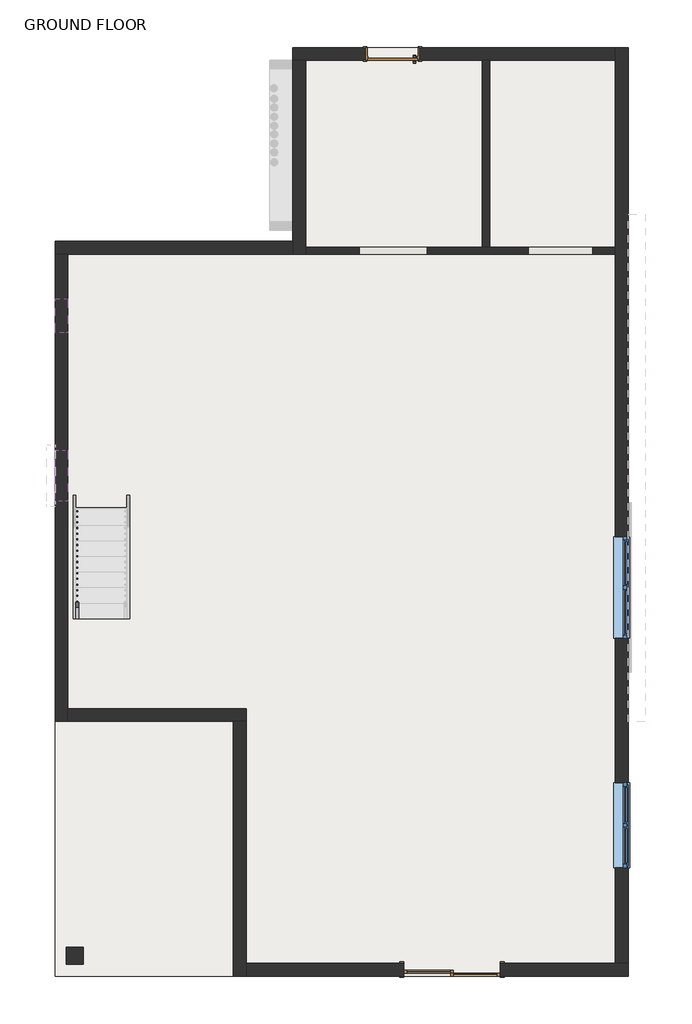
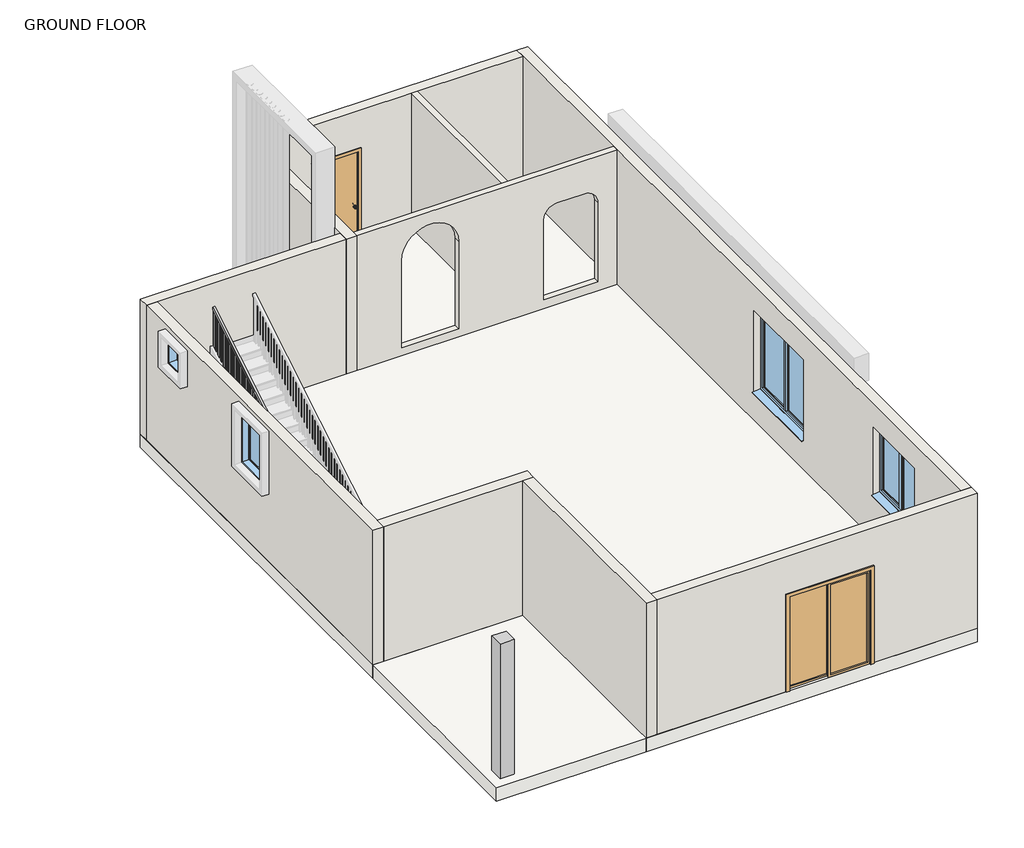
# One storey, part 1 of 2: 10 walls, 4 windows, 2 doors, 2 slabs, 1 column, 1 railing.
"""IFC4 building model written with IfcOpenShell, lengths in millimetres."""

from ifc_helpers import new_model, si_unit, frame, origin, origin_with_axes, place, context, project, spatial, polyline, circle_curve, outline, extrude, faceted_brep, transform, mapped, element, save
from ifc_brep_helpers import plane_surface, revolved_surface, advanced_brep
from components import rectangular_column_1_x_1_columns_77852fec, door_45189e27, door_1d7b229f, window_80340324, fixed_window_3_x_3_dcb239d8, w2_6_x_6_window_82e362f5, w2_windows_5_x_5_8ac21896

model = new_model("IFC4")

# Units and contexts
model_context = context("Model", 3, world=origin())
ifc_project = project(units=[si_unit("LENGTHUNIT", "METRE", prefix="MILLI")], contexts=[model_context])

# Site, building, storey
site = spatial("IfcSite", under=ifc_project)
building = spatial("IfcBuilding", under=site)
storey = spatial("IfcBuildingStorey", under=building, Name="GROUND FLOOR", Elevation=304.8)

# Column
placement = place(None, origin())
rectangular_column_1_x_1_columns_shape = rectangular_column_1_x_1_columns_77852fec(model_context)
element("IfcColumn", 1, ObjectType="Rectangular Column : 1' x 1' columns", at=placement, inside=storey, context=model_context, shape_type="MappedRepresentation", body=[
    mapped(rectangular_column_1_x_1_columns_shape, transform((-5747.4727592, -4033.4659376, 0.0), x_axis=(1.0, 0.0, 0.0), y_axis=(0.0, 1.0, 0.0), z_axis=(0.0, 0.0, 1.0))),
])

# Doors
door_shape = door_45189e27(model_context)
element("IfcDoor", 2, ObjectType="Door-Double-Sliding : 68\" x 84\"", at=placement, inside=storey, context=model_context, shape_type="MappedRepresentation", body=[
    mapped(door_shape, transform((1027.2719693, -4152.8358748, 304.8), x_axis=(-1.0, 0.0, 0.0), y_axis=(0.0, -1.0, 0.0), z_axis=(0.0, 0.0, 1.0))),
])
door_2_shape = door_1d7b229f(model_context)
element("IfcDoor", 3, ObjectType="Door-Interior-Single-Flush_Panel-Wood : 36\" x 84\"", at=placement, inside=storey, context=model_context, shape_type="MappedRepresentation", body=[
    mapped(door_2_shape, transform((-39.5280307, 12150.7891252, 304.8), x_axis=(-1.0, 0.0, 0.0), y_axis=(0.0, -1.0, 0.0), z_axis=(0.0, 0.0, 1.0))),
])

# Railing
element("IfcRailing", 4, ObjectType="Handrail - Rectangular", at=placement, inside=storey, context=model_context, shape_type="SweptSolid", body=[
    extrude(outline(polyline([(2020.7325341, 1329.1318731), (2020.7325341, 1388.5333333), (6770.5325341, 4267.2), (6770.5325341, 4207.7985397), (2020.7325341, 1329.1318731)])), frame((-5721.5875748, 0.0, 0.0), z_axis=(1.0, 0.0, 0.0), x_axis=(0.0, 1.0, 0.0)), (0.0, 0.0, 1.0), 50.8),
    extrude(outline(polyline([(6703.8575341, 4167.3894488), (6703.8575341, 3183.4666667), (6684.8075341, 3183.4666667), (6684.8075341, 4155.8439943), (6703.8575341, 4167.3894488)])), frame((-5705.7125748, 0.0, 0.0), z_axis=(1.0, 0.0, 0.0), x_axis=(0.0, 1.0, 0.0)), (0.0, 0.0, 1.0), 19.05),
    extrude(outline(polyline([(6602.2575341, 4105.8136913), (6602.2575341, 3183.4666667), (6583.2075341, 3183.4666667), (6583.2075341, 4094.2682367), (6602.2575341, 4105.8136913)])), frame((-5705.7125748, 0.0, 0.0), z_axis=(1.0, 0.0, 0.0), x_axis=(0.0, 1.0, 0.0)), (0.0, 0.0, 1.0), 19.05),
    extrude(outline(polyline([(6500.6575341, 4044.2379337), (6500.6575341, 3183.4666667), (6481.6075341, 3183.4666667), (6481.6075341, 4032.6924791), (6500.6575341, 4044.2379337)])), frame((-5705.7125748, 0.0, 0.0), z_axis=(1.0, 0.0, 0.0), x_axis=(0.0, 1.0, 0.0)), (0.0, 0.0, 1.0), 19.05),
    extrude(outline(polyline([(6399.0575341, 3982.6621761), (6399.0575341, 3014.1333333), (6380.0075341, 3014.1333333), (6380.0075341, 3971.1167216), (6399.0575341, 3982.6621761)])), frame((-5705.7125748, 0.0, 0.0), z_axis=(1.0, 0.0, 0.0), x_axis=(0.0, 1.0, 0.0)), (0.0, 0.0, 1.0), 19.05),
    extrude(outline(polyline([(6297.4575341, 3921.0864185), (6297.4575341, 3014.1333333), (6278.4075341, 3014.1333333), (6278.4075341, 3909.540964), (6297.4575341, 3921.0864185)])), frame((-5705.7125748, 0.0, 0.0), z_axis=(1.0, 0.0, 0.0), x_axis=(0.0, 1.0, 0.0)), (0.0, 0.0, 1.0), 19.05),
    extrude(outline(polyline([(6195.8575341, 3859.510661), (6195.8575341, 2844.8), (6176.8075341, 2844.8), (6176.8075341, 3847.9652064), (6195.8575341, 3859.510661)])), frame((-5705.7125748, 0.0, 0.0), z_axis=(1.0, 0.0, 0.0), x_axis=(0.0, 1.0, 0.0)), (0.0, 0.0, 1.0), 19.05),
    extrude(outline(polyline([(6094.2575341, 3797.9349034), (6094.2575341, 2844.8), (6075.2075341, 2844.8), (6075.2075341, 3786.3894488), (6094.2575341, 3797.9349034)])), frame((-5705.7125748, 0.0, 0.0), z_axis=(1.0, 0.0, 0.0), x_axis=(0.0, 1.0, 0.0)), (0.0, 0.0, 1.0), 19.05),
    extrude(outline(polyline([(5992.6575341, 3736.3591458), (5992.6575341, 2844.8), (5973.6075341, 2844.8), (5973.6075341, 3724.8136913), (5992.6575341, 3736.3591458)])), frame((-5705.7125748, 0.0, 0.0), z_axis=(1.0, 0.0, 0.0), x_axis=(0.0, 1.0, 0.0)), (0.0, 0.0, 1.0), 19.05),
    extrude(outline(polyline([(5891.0575341, 3674.7833882), (5891.0575341, 2675.4666667), (5872.0075341, 2675.4666667), (5872.0075341, 3663.2379337), (5891.0575341, 3674.7833882)])), frame((-5705.7125748, 0.0, 0.0), z_axis=(1.0, 0.0, 0.0), x_axis=(0.0, 1.0, 0.0)), (0.0, 0.0, 1.0), 19.05),
    extrude(outline(polyline([(5789.4575341, 3613.2076307), (5789.4575341, 2675.4666667), (5770.4075341, 2675.4666667), (5770.4075341, 3601.6621761), (5789.4575341, 3613.2076307)])), frame((-5705.7125748, 0.0, 0.0), z_axis=(1.0, 0.0, 0.0), x_axis=(0.0, 1.0, 0.0)), (0.0, 0.0, 1.0), 19.05),
    extrude(outline(polyline([(5687.8575341, 3551.6318731), (5687.8575341, 2675.4666667), (5668.8075341, 2675.4666667), (5668.8075341, 3540.0864185), (5687.8575341, 3551.6318731)])), frame((-5705.7125748, 0.0, 0.0), z_axis=(1.0, 0.0, 0.0), x_axis=(0.0, 1.0, 0.0)), (0.0, 0.0, 1.0), 19.05),
    extrude(outline(polyline([(5586.2575341, 3490.0561155), (5586.2575341, 2506.1333333), (5567.2075341, 2506.1333333), (5567.2075341, 3478.510661), (5586.2575341, 3490.0561155)])), frame((-5705.7125748, 0.0, 0.0), z_axis=(1.0, 0.0, 0.0), x_axis=(0.0, 1.0, 0.0)), (0.0, 0.0, 1.0), 19.05),
    extrude(outline(polyline([(5484.6575341, 3428.4803579), (5484.6575341, 2506.1333333), (5465.6075341, 2506.1333333), (5465.6075341, 3416.9349034), (5484.6575341, 3428.4803579)])), frame((-5705.7125748, 0.0, 0.0), z_axis=(1.0, 0.0, 0.0), x_axis=(0.0, 1.0, 0.0)), (0.0, 0.0, 1.0), 19.05),
    extrude(outline(polyline([(5383.0575341, 3366.9046004), (5383.0575341, 2506.1333333), (5364.0075341, 2506.1333333), (5364.0075341, 3355.3591458), (5383.0575341, 3366.9046004)])), frame((-5705.7125748, 0.0, 0.0), z_axis=(1.0, 0.0, 0.0), x_axis=(0.0, 1.0, 0.0)), (0.0, 0.0, 1.0), 19.05),
    extrude(outline(polyline([(5281.4575341, 3305.3288428), (5281.4575341, 2336.8), (5262.4075341, 2336.8), (5262.4075341, 3293.7833882), (5281.4575341, 3305.3288428)])), frame((-5705.7125748, 0.0, 0.0), z_axis=(1.0, 0.0, 0.0), x_axis=(0.0, 1.0, 0.0)), (0.0, 0.0, 1.0), 19.05),
    extrude(outline(polyline([(5179.8575341, 3243.7530852), (5179.8575341, 2336.8), (5160.8075341, 2336.8), (5160.8075341, 3232.2076307), (5179.8575341, 3243.7530852)])), frame((-5705.7125748, 0.0, 0.0), z_axis=(1.0, 0.0, 0.0), x_axis=(0.0, 1.0, 0.0)), (0.0, 0.0, 1.0), 19.05),
    extrude(outline(polyline([(5078.2575341, 3182.1773276), (5078.2575341, 2167.4666667), (5059.2075341, 2167.4666667), (5059.2075341, 3170.6318731), (5078.2575341, 3182.1773276)])), frame((-5705.7125748, 0.0, 0.0), z_axis=(1.0, 0.0, 0.0), x_axis=(0.0, 1.0, 0.0)), (0.0, 0.0, 1.0), 19.05),
    extrude(outline(polyline([(4976.6575341, 3120.60157), (4976.6575341, 2167.4666667), (4957.6075341, 2167.4666667), (4957.6075341, 3109.0561155), (4976.6575341, 3120.60157)])), frame((-5705.7125748, 0.0, 0.0), z_axis=(1.0, 0.0, 0.0), x_axis=(0.0, 1.0, 0.0)), (0.0, 0.0, 1.0), 19.05),
    extrude(outline(polyline([(4875.0575341, 3059.0258125), (4875.0575341, 2167.4666667), (4856.0075341, 2167.4666667), (4856.0075341, 3047.4803579), (4875.0575341, 3059.0258125)])), frame((-5705.7125748, 0.0, 0.0), z_axis=(1.0, 0.0, 0.0), x_axis=(0.0, 1.0, 0.0)), (0.0, 0.0, 1.0), 19.05),
    extrude(outline(polyline([(4773.4575341, 2997.4500549), (4773.4575341, 1998.1333333), (4754.4075341, 1998.1333333), (4754.4075341, 2985.9046004), (4773.4575341, 2997.4500549)])), frame((-5705.7125748, 0.0, 0.0), z_axis=(1.0, 0.0, 0.0), x_axis=(0.0, 1.0, 0.0)), (0.0, 0.0, 1.0), 19.05),
    extrude(outline(polyline([(4671.8575341, 2935.8742973), (4671.8575341, 1998.1333333), (4652.8075341, 1998.1333333), (4652.8075341, 2924.3288428), (4671.8575341, 2935.8742973)])), frame((-5705.7125748, 0.0, 0.0), z_axis=(1.0, 0.0, 0.0), x_axis=(0.0, 1.0, 0.0)), (0.0, 0.0, 1.0), 19.05),
    extrude(outline(polyline([(4570.2575341, 2874.2985397), (4570.2575341, 1998.1333333), (4551.2075341, 1998.1333333), (4551.2075341, 2862.7530852), (4570.2575341, 2874.2985397)])), frame((-5705.7125748, 0.0, 0.0), z_axis=(1.0, 0.0, 0.0), x_axis=(0.0, 1.0, 0.0)), (0.0, 0.0, 1.0), 19.05),
    extrude(outline(polyline([(4468.6575341, 2812.7227822), (4468.6575341, 1828.8), (4449.6075341, 1828.8), (4449.6075341, 2801.1773276), (4468.6575341, 2812.7227822)])), frame((-5705.7125748, 0.0, 0.0), z_axis=(1.0, 0.0, 0.0), x_axis=(0.0, 1.0, 0.0)), (0.0, 0.0, 1.0), 19.05),
    extrude(outline(polyline([(4367.0575341, 2751.1470246), (4367.0575341, 1828.8), (4348.0075341, 1828.8), (4348.0075341, 2739.60157), (4367.0575341, 2751.1470246)])), frame((-5705.7125748, 0.0, 0.0), z_axis=(1.0, 0.0, 0.0), x_axis=(0.0, 1.0, 0.0)), (0.0, 0.0, 1.0), 19.05),
    extrude(outline(polyline([(4265.4575341, 2689.571267), (4265.4575341, 1828.8), (4246.4075341, 1828.8), (4246.4075341, 2678.0258125), (4265.4575341, 2689.571267)])), frame((-5705.7125748, 0.0, 0.0), z_axis=(1.0, 0.0, 0.0), x_axis=(0.0, 1.0, 0.0)), (0.0, 0.0, 1.0), 19.05),
    extrude(outline(polyline([(4163.8575341, 2627.9955094), (4163.8575341, 1659.4666667), (4144.8075341, 1659.4666667), (4144.8075341, 2616.4500549), (4163.8575341, 2627.9955094)])), frame((-5705.7125748, 0.0, 0.0), z_axis=(1.0, 0.0, 0.0), x_axis=(0.0, 1.0, 0.0)), (0.0, 0.0, 1.0), 19.05),
    extrude(outline(polyline([(4062.2575341, 2566.4197519), (4062.2575341, 1659.4666667), (4043.2075341, 1659.4666667), (4043.2075341, 2554.8742973), (4062.2575341, 2566.4197519)])), frame((-5705.7125748, 0.0, 0.0), z_axis=(1.0, 0.0, 0.0), x_axis=(0.0, 1.0, 0.0)), (0.0, 0.0, 1.0), 19.05),
    extrude(outline(polyline([(3960.6575341, 2504.8439943), (3960.6575341, 1490.1333333), (3941.6075341, 1490.1333333), (3941.6075341, 2493.2985397), (3960.6575341, 2504.8439943)])), frame((-5705.7125748, 0.0, 0.0), z_axis=(1.0, 0.0, 0.0), x_axis=(0.0, 1.0, 0.0)), (0.0, 0.0, 1.0), 19.05),
    extrude(outline(polyline([(3859.0575341, 2443.2682367), (3859.0575341, 1490.1333333), (3840.0075341, 1490.1333333), (3840.0075341, 2431.7227822), (3859.0575341, 2443.2682367)])), frame((-5705.7125748, 0.0, 0.0), z_axis=(1.0, 0.0, 0.0), x_axis=(0.0, 1.0, 0.0)), (0.0, 0.0, 1.0), 19.05),
    extrude(outline(polyline([(3757.4575341, 2381.6924791), (3757.4575341, 1490.1333333), (3738.4075341, 1490.1333333), (3738.4075341, 2370.1470246), (3757.4575341, 2381.6924791)])), frame((-5705.7125748, 0.0, 0.0), z_axis=(1.0, 0.0, 0.0), x_axis=(0.0, 1.0, 0.0)), (0.0, 0.0, 1.0), 19.05),
    extrude(outline(polyline([(3655.8575341, 2320.1167216), (3655.8575341, 1320.8), (3636.8075341, 1320.8), (3636.8075341, 2308.571267), (3655.8575341, 2320.1167216)])), frame((-5705.7125748, 0.0, 0.0), z_axis=(1.0, 0.0, 0.0), x_axis=(0.0, 1.0, 0.0)), (0.0, 0.0, 1.0), 19.05),
    extrude(outline(polyline([(3554.2575341, 2258.540964), (3554.2575341, 1320.8), (3535.2075341, 1320.8), (3535.2075341, 2246.9955094), (3554.2575341, 2258.540964)])), frame((-5705.7125748, 0.0, 0.0), z_axis=(1.0, 0.0, 0.0), x_axis=(0.0, 1.0, 0.0)), (0.0, 0.0, 1.0), 19.05),
    extrude(outline(polyline([(3452.6575341, 2196.9652064), (3452.6575341, 1320.8), (3433.6075341, 1320.8), (3433.6075341, 2185.4197519), (3452.6575341, 2196.9652064)])), frame((-5705.7125748, 0.0, 0.0), z_axis=(1.0, 0.0, 0.0), x_axis=(0.0, 1.0, 0.0)), (0.0, 0.0, 1.0), 19.05),
    extrude(outline(polyline([(3351.0575341, 2135.3894488), (3351.0575341, 1151.4666667), (3332.0075341, 1151.4666667), (3332.0075341, 2123.8439943), (3351.0575341, 2135.3894488)])), frame((-5705.7125748, 0.0, 0.0), z_axis=(1.0, 0.0, 0.0), x_axis=(0.0, 1.0, 0.0)), (0.0, 0.0, 1.0), 19.05),
    extrude(outline(polyline([(3249.4575341, 2073.8136913), (3249.4575341, 1151.4666667), (3230.4075341, 1151.4666667), (3230.4075341, 2062.2682367), (3249.4575341, 2073.8136913)])), frame((-5705.7125748, 0.0, 0.0), z_axis=(1.0, 0.0, 0.0), x_axis=(0.0, 1.0, 0.0)), (0.0, 0.0, 1.0), 19.05),
    extrude(outline(polyline([(3147.8575341, 2012.2379337), (3147.8575341, 1151.4666667), (3128.8075341, 1151.4666667), (3128.8075341, 2000.6924791), (3147.8575341, 2012.2379337)])), frame((-5705.7125748, 0.0, 0.0), z_axis=(1.0, 0.0, 0.0), x_axis=(0.0, 1.0, 0.0)), (0.0, 0.0, 1.0), 19.05),
    extrude(outline(polyline([(3046.2575341, 1950.6621761), (3046.2575341, 982.1333333), (3027.2075341, 982.1333333), (3027.2075341, 1939.1167216), (3046.2575341, 1950.6621761)])), frame((-5705.7125748, 0.0, 0.0), z_axis=(1.0, 0.0, 0.0), x_axis=(0.0, 1.0, 0.0)), (0.0, 0.0, 1.0), 19.05),
    extrude(outline(polyline([(2944.6575341, 1889.0864185), (2944.6575341, 982.1333333), (2925.6075341, 982.1333333), (2925.6075341, 1877.540964), (2944.6575341, 1889.0864185)])), frame((-5705.7125748, 0.0, 0.0), z_axis=(1.0, 0.0, 0.0), x_axis=(0.0, 1.0, 0.0)), (0.0, 0.0, 1.0), 19.05),
    extrude(outline(polyline([(2843.0575341, 1827.510661), (2843.0575341, 812.8), (2824.0075341, 812.8), (2824.0075341, 1815.9652064), (2843.0575341, 1827.510661)])), frame((-5705.7125748, 0.0, 0.0), z_axis=(1.0, 0.0, 0.0), x_axis=(0.0, 1.0, 0.0)), (0.0, 0.0, 1.0), 19.05),
    extrude(outline(polyline([(2741.4575341, 1765.9349034), (2741.4575341, 812.8), (2722.4075341, 812.8), (2722.4075341, 1754.3894488), (2741.4575341, 1765.9349034)])), frame((-5705.7125748, 0.0, 0.0), z_axis=(1.0, 0.0, 0.0), x_axis=(0.0, 1.0, 0.0)), (0.0, 0.0, 1.0), 19.05),
    extrude(outline(polyline([(2639.8575341, 1704.3591458), (2639.8575341, 812.8), (2620.8075341, 812.8), (2620.8075341, 1692.8136913), (2639.8575341, 1704.3591458)])), frame((-5705.7125748, 0.0, 0.0), z_axis=(1.0, 0.0, 0.0), x_axis=(0.0, 1.0, 0.0)), (0.0, 0.0, 1.0), 19.05),
    extrude(outline(polyline([(2538.2575341, 1642.7833882), (2538.2575341, 643.4666667), (2519.2075341, 643.4666667), (2519.2075341, 1631.2379337), (2538.2575341, 1642.7833882)])), frame((-5705.7125748, 0.0, 0.0), z_axis=(1.0, 0.0, 0.0), x_axis=(0.0, 1.0, 0.0)), (0.0, 0.0, 1.0), 19.05),
    extrude(outline(polyline([(2436.6575341, 1581.2076307), (2436.6575341, 643.4666667), (2417.6075341, 643.4666667), (2417.6075341, 1569.6621761), (2436.6575341, 1581.2076307)])), frame((-5705.7125748, 0.0, 0.0), z_axis=(1.0, 0.0, 0.0), x_axis=(0.0, 1.0, 0.0)), (0.0, 0.0, 1.0), 19.05),
    extrude(outline(polyline([(2335.0575341, 1519.6318731), (2335.0575341, 643.4666667), (2316.0075341, 643.4666667), (2316.0075341, 1508.0864185), (2335.0575341, 1519.6318731)])), frame((-5705.7125748, 0.0, 0.0), z_axis=(1.0, 0.0, 0.0), x_axis=(0.0, 1.0, 0.0)), (0.0, 0.0, 1.0), 19.05),
    extrude(outline(polyline([(2233.4575341, 1458.0561155), (2233.4575341, 474.1333333), (2214.4075341, 474.1333333), (2214.4075341, 1446.510661), (2233.4575341, 1458.0561155)])), frame((-5705.7125748, 0.0, 0.0), z_axis=(1.0, 0.0, 0.0), x_axis=(0.0, 1.0, 0.0)), (0.0, 0.0, 1.0), 19.05),
    extrude(outline(polyline([(2131.8575341, 1396.4803579), (2131.8575341, 474.1333333), (2112.8075341, 474.1333333), (2112.8075341, 1384.9349034), (2131.8575341, 1396.4803579)])), frame((-5705.7125748, 0.0, 0.0), z_axis=(1.0, 0.0, 0.0), x_axis=(0.0, 1.0, 0.0)), (0.0, 0.0, 1.0), 19.05),
    extrude(outline(polyline([(6770.5325341, 4207.7985397), (6770.5325341, 3183.4666667), (6751.4825341, 3183.4666667), (6751.4825341, 4196.2530852), (6770.5325341, 4207.7985397)])), frame((-5705.7125748, 0.0, 0.0), z_axis=(1.0, 0.0, 0.0), x_axis=(0.0, 1.0, 0.0)), (0.0, 0.0, 1.0), 19.05),
    extrude(outline(polyline([(2039.7825341, 1340.6773276), (2039.7825341, 474.1333333), (2020.7325341, 474.1333333), (2020.7325341, 1329.1318731), (2039.7825341, 1340.6773276)])), frame((-5705.7125748, 0.0, 0.0), z_axis=(1.0, 0.0, 0.0), x_axis=(0.0, 1.0, 0.0)), (0.0, 0.0, 1.0), 19.05),
])

# Slabs
element("IfcSlab", 5, ObjectType="MARBLE 1'", at=placement, inside=storey, context=model_context, shape_type="SweptSolid", body=[
    extrude(outline(polyline([(4189.5719693, 12268.2641252), (4189.5719693, -4394.1358748), (-2897.0280307, -4394.1358748), (-2897.0280307, 177.8641252), (-6097.4280307, 177.8641252), (-6097.4280307, 8788.4641252), (-1830.2280307, 8788.4641252), (-1830.2280307, 12268.2641252), (4189.5719693, 12268.2641252)])), origin_with_axes(), (0.0, 0.0, 1.0), 304.8),
])
element("IfcSlab", 6, ObjectType="MARBLE 1'", at=placement, inside=storey, context=model_context, shape_type="SweptSolid", body=[
    extrude(outline(polyline([(-2897.0280307, 177.8641252), (-2897.0280307, -4394.1358748), (-6097.4280307, -4394.1358748), (-6097.4280307, 177.8641252), (-2897.0280307, 177.8641252)])), origin_with_axes(), (0.0, 0.0, 1.0), 304.8),
])

# Walls
element("IfcWall", 7, ObjectType="INNER WALL5\"", at=placement, inside=storey, context=model_context, shape_type="SweptSolid", body=[
    extrude(outline(polyline([(1573.3719693, 8686.8641252), (1573.3719693, 12039.6641252), (1700.3719693, 12039.6641252), (1700.3719693, 8686.8641252), (1573.3719693, 8686.8641252)])), frame((0.0, 0.0, 304.8), z_axis=(0.0, 0.0, 1.0), x_axis=(1.0, 0.0, 0.0)), (0.0, 0.0, 1.0), 3048.0),
])
element("IfcWall", 8, ObjectType="INNER WALL5\"", at=placement, inside=storey, context=model_context, shape_type="AdvancedBrep", body=[
    advanced_brep(
    [(-1601.6280307, 8559.8641252, 304.8), (3960.9719693, 8559.8641252, 304.8), (3960.9719693, 8559.8641252, 3352.8), (-1601.6280307, 8559.8641252, 3352.8), (578.4377275, 8559.8641252, 482.354064), (-640.7622725, 8559.8641252, 482.354064), (-640.7622725, 8559.8641252, 2453.5766961), (578.4377275, 8559.8641252, 2453.5766961), (3553.6199856, 8559.8641252, 505.817995), (2397.9199856, 8559.8641252, 505.817995), (2397.9199856, 8559.8641252, 2315.4306081), (2677.4573726, 8559.8641252, 2594.967995), (3248.8199856, 8559.8641252, 2594.967995), (3553.6199856, 8559.8641252, 2290.167995), (-1601.6280307, 8686.8641252, 304.8), (-1601.6280307, 8686.8641252, 3352.8), (1573.3719693, 8686.8641252, 3352.8), (1700.3719693, 8686.8641252, 3352.8), (3960.9719693, 8686.8641252, 3352.8), (3960.9719693, 8686.8641252, 304.8), (1700.3719693, 8686.8641252, 304.8), (1573.3719693, 8686.8641252, 304.8), (578.4377275, 8686.8641252, 482.354064), (578.4377275, 8686.8641252, 2453.5766961), (-640.7622725, 8686.8641252, 2453.5766961), (-640.7622725, 8686.8641252, 482.354064), (3553.6199856, 8686.8641252, 505.817995), (3553.6199856, 8686.8641252, 2290.167995), (3248.8199856, 8686.8641252, 2594.967995), (2677.4573726, 8686.8641252, 2594.967995), (2397.9199856, 8686.8641252, 2315.4306081), (2397.9199856, 8686.8641252, 505.817995)],
    [
        (0, 1),
        (1, 2),
        (2, 3),
        (3, 0),
        (4, 5),
        (5, 6),
        (6, 7, circle_curve(frame((-31.1622725, 8559.8641252, 2453.5766961), z_axis=(0.0, 1.0, 0.0), x_axis=(-1.0, 0.0, 0.0)), 609.6)),
        (7, 4),
        (8, 9),
        (9, 10),
        (10, 11, circle_curve(frame((2677.4573726, 8559.8641252, 2315.4306081), z_axis=(0.0, 1.0, 0.0), x_axis=(-1.0, 0.0, 0.0)), 279.5373869)),
        (11, 12),
        (12, 13, circle_curve(frame((3248.8199856, 8559.8641252, 2290.167995), z_axis=(0.0, 1.0, 0.0), x_axis=(-1.0, 0.0, 0.0)), 304.8)),
        (13, 8),
        (14, 15),
        (15, 16),
        (16, 17),
        (17, 18),
        (18, 19),
        (19, 20),
        (20, 21),
        (21, 14),
        (22, 23),
        (23, 24, circle_curve(frame((-31.1622725, 8686.8641252, 2453.5766961), z_axis=(0.0, -1.0, 0.0), x_axis=(-1.0, 0.0, 0.0)), 609.6)),
        (24, 25),
        (25, 22),
        (26, 27),
        (27, 28, circle_curve(frame((3248.8199856, 8686.8641252, 2290.167995), z_axis=(0.0, -1.0, 0.0), x_axis=(-1.0, 0.0, 0.0)), 304.8)),
        (28, 29),
        (29, 30, circle_curve(frame((2677.4573726, 8686.8641252, 2315.4306081), z_axis=(0.0, -1.0, 0.0), x_axis=(-1.0, 0.0, 0.0)), 279.5373869)),
        (30, 31),
        (31, 26),
        (1, 19),
        (18, 2),
        (3, 15),
        (14, 0),
        (4, 22),
        (25, 5),
        (24, 6),
        (23, 7),
        (8, 26),
        (31, 9),
        (30, 10),
        (29, 11),
        (28, 12),
        (27, 13),
    ],
    [
        plane_surface(frame((-5564.0280307, 8559.8641252, 304.8), z_axis=(0.0, -1.0, 0.0), x_axis=(1.0, 0.0, 0.0))),
        plane_surface(frame((-5564.0280307, 8686.8641252, 304.8), z_axis=(0.0, 1.0, 0.0), x_axis=(-1.0, 0.0, 0.0))),
        plane_surface(frame((3960.9719693, -1384.2358748, 304.8), z_axis=(1.0, 0.0, 0.0), x_axis=(0.0, -1.0, 0.0))),
        plane_surface(frame((-1601.6280307, 11722.1641252, 304.8), z_axis=(-1.0, 0.0, 0.0), x_axis=(0.0, 1.0, 0.0))),
        plane_surface(frame((-1715.9280307, 8559.8641252, 304.8), z_axis=(0.0, 0.0, -1.0), x_axis=(0.0, 1.0, 0.0))),
        plane_surface(frame((4075.2719693, 8559.8641252, 3352.8), z_axis=(0.0, 0.0, 1.0), x_axis=(0.0, 1.0, 0.0))),
        plane_surface(frame((578.4377275, 8559.8641252, 482.354064), z_axis=(0.0, 0.0, 1.0), x_axis=(0.0, 1.0, 0.0))),
        plane_surface(frame((-640.7622725, 8559.8641252, 482.354064), z_axis=(1.0, 0.0, 0.0), x_axis=(0.0, 1.0, 0.0))),
        revolved_surface(polyline([(-640.7622725, 8686.8641252, 2453.5766961), (-640.7622725, 8559.8641252, 2453.5766961)]), (-31.1622725, 8623.3641252, 2453.5766961), (0.0, 1.0, 0.0)),
        plane_surface(frame((578.4377275, 8559.8641252, 2453.5766961), z_axis=(-1.0, 0.0, 0.0), x_axis=(0.0, 1.0, 0.0))),
        plane_surface(frame((3553.6199856, 8559.8641252, 505.817995), z_axis=(0.0, 0.0, 1.0), x_axis=(0.0, 1.0, 0.0))),
        plane_surface(frame((2397.9199856, 8559.8641252, 505.817995), z_axis=(1.0, 0.0, 0.0), x_axis=(0.0, 1.0, 0.0))),
        revolved_surface(polyline([(2397.9199857, 8686.8641252, 2315.4306081), (2397.9199857, 8559.8641252, 2315.4306081)]), (2677.4573726, 8623.3641252, 2315.4306081), (0.0, 1.0, 0.0)),
        plane_surface(frame((2677.4573726, 8559.8641252, 2594.967995), z_axis=(0.0, 0.0, -1.0), x_axis=(0.0, 1.0, 0.0))),
        revolved_surface(polyline([(2944.0199856, 8686.8641252, 2290.167995), (2944.0199856, 8559.8641252, 2290.167995)]), (3248.8199856, 8623.3641252, 2290.167995), (0.0, 1.0, 0.0)),
        plane_surface(frame((3553.6199856, 8559.8641252, 2290.167995), z_axis=(-1.0, 0.0, 0.0), x_axis=(0.0, 1.0, 0.0))),
    ],
    [
        (0, [[1, 2, 3, 4], [5, 6, 7, 8], [9, 10, 11, 12, 13, 14]]),
        (1, [[15, 16, 17, 18, 19, 20, 21, 22], [23, 24, 25, 26], [27, 28, 29, 30, 31, 32]]),
        (2, [[-2, 33, -19, 34]]),
        (3, [[-4, 35, -15, 36]]),
        (4, [[-1, -36, -22, -21, -20, -33]]),
        (5, [[-3, -34, -18, -17, -16, -35]]),
        (6, [[-5, 37, -26, 38]]),
        (7, [[-6, -38, -25, 39]]),
        (8, [[-7, -39, -24, 40]]),
        (9, [[-8, -40, -23, -37]]),
        (10, [[-9, 41, -32, 42]]),
        (11, [[-10, -42, -31, 43]]),
        (12, [[-11, -43, -30, 44]]),
        (13, [[-12, -44, -29, 45]]),
        (14, [[-13, -45, -28, 46]]),
        (15, [[-14, -46, -27, -41]]),
    ],
),
])
element("IfcWall", 9, ObjectType="OUTER WALL 9\"", at=placement, inside=storey, context=model_context, shape_type="Brep", body=[
    faceted_brep([(4189.5719693, -4165.5358748, 304.8), (4189.5719693, 12268.2641252, 304.8), (4189.5719693, 12268.2641252, 3352.8), (4189.5719693, -4165.5358748, 3352.8), (4189.5719693, 1663.7641252, 949.2), (4189.5719693, 1663.7641252, 2778.0), (4189.5719693, 3492.5641252, 2778.0), (4189.5719693, 3492.5641252, 949.2), (4189.5719693, -2451.0358748, 1304.8), (4189.5719693, -2451.0358748, 2828.8), (4189.5719693, -927.0358748, 2828.8), (4189.5719693, -927.0358748, 1304.8), (3960.9719693, -4165.5358748, 304.8), (3960.9719693, -4165.5358748, 3352.8), (3960.9719693, 8559.8641252, 3352.8), (3960.9719693, 8686.8641252, 3352.8), (3960.9719693, 12039.6641252, 3352.8), (3960.9719693, 12268.2641252, 3352.8), (3960.9719693, 12268.2641252, 304.8), (3960.9719693, 12039.6641252, 304.8), (3960.9719693, 8686.8641252, 304.8), (3960.9719693, 8559.8641252, 304.8), (3960.9719693, 1663.7641252, 949.2), (3960.9719693, 3492.5641252, 949.2), (3960.9719693, 3492.5641252, 2778.0), (3960.9719693, 1663.7641252, 2778.0), (3960.9719693, -2451.0358748, 1304.8), (3960.9719693, -927.0358748, 1304.8), (3960.9719693, -927.0358748, 2828.8), (3960.9719693, -2451.0358748, 2828.8)], [[[0, 1, 2, 3], [4, 5, 6, 7], [8, 9, 10, 11]], [[12, 13, 14, 15, 16, 17, 18, 19, 20, 21], [22, 23, 24, 25], [26, 27, 28, 29]], [[1, 0, 12, 21, 20, 19, 18]], [[3, 2, 17, 16, 15, 14, 13]], [[2, 1, 18, 17]], [[0, 3, 13, 12]], [[5, 4, 22, 25]], [[6, 5, 25, 24]], [[7, 6, 24, 23]], [[4, 7, 23, 22]], [[9, 8, 26, 29]], [[10, 9, 29, 28]], [[11, 10, 28, 27]], [[8, 11, 27, 26]]]),
])
element("IfcWall", 10, ObjectType="OUTER WALL 9\"", at=placement, inside=storey, context=model_context, shape_type="Brep", body=[
    faceted_brep([(-1830.2280307, 12268.2641252, 3352.8), (3960.9719693, 12268.2641252, 3352.8), (3960.9719693, 12268.2641252, 304.8), (443.0719693, 12268.2641252, 304.8), (443.0719693, 12268.2641252, 2463.8), (-522.1280307, 12268.2641252, 2463.8), (-522.1280307, 12268.2641252, 304.8), (-1830.2280307, 12268.2641252, 304.8), (3960.9719693, 12039.6641252, 3352.8), (1700.3719693, 12039.6641252, 3352.8), (1573.3719693, 12039.6641252, 3352.8), (-1601.6280307, 12039.6641252, 3352.8), (-1830.2280307, 12039.6641252, 3352.8), (-1830.2280307, 12039.6641252, 304.8), (-1601.6280307, 12039.6641252, 304.8), (-522.1280307, 12039.6641252, 304.8), (-522.1280307, 12039.6641252, 2463.8), (443.0719693, 12039.6641252, 2463.8), (443.0719693, 12039.6641252, 304.8), (1573.3719693, 12039.6641252, 304.8), (1700.3719693, 12039.6641252, 304.8), (3960.9719693, 12039.6641252, 304.8)], [[[0, 1, 2, 3, 4, 5, 6, 7]], [[8, 9, 10, 11, 12, 13, 14, 15, 16, 17, 18, 19, 20, 21]], [[2, 21, 20, 19, 18, 3]], [[13, 7, 6, 15, 14]], [[1, 0, 12, 11, 10, 9, 8]], [[2, 1, 8, 21]], [[0, 7, 13, 12]], [[5, 16, 15, 6]], [[16, 5, 4, 17]], [[17, 4, 3, 18]]]),
])
element("IfcWall", 11, ObjectType="OUTER WALL 9\"", at=placement, inside=storey, context=model_context, shape_type="Brep", body=[
    faceted_brep([(-1830.2280307, 12039.6641252, 304.8), (-1830.2280307, 8788.4641252, 304.8), (-1830.2280307, 8559.8641252, 304.8), (-1830.2280307, 8559.8641252, 3352.8), (-1830.2280307, 8788.4641252, 3352.8), (-1830.2280307, 12039.6641252, 3352.8), (-1601.6280307, 12039.6641252, 304.8), (-1601.6280307, 12039.6641252, 3352.8), (-1601.6280307, 8686.8641252, 3352.8), (-1601.6280307, 8559.8641252, 3352.8), (-1601.6280307, 8559.8641252, 304.8), (-1601.6280307, 8686.8641252, 304.8)], [[[0, 1, 2, 3, 4, 5]], [[6, 7, 8, 9, 10, 11]], [[2, 1, 0, 6, 11, 10]], [[5, 4, 3, 9, 8, 7]], [[0, 5, 7, 6]], [[3, 2, 10, 9]]]),
])
element("IfcWall", 12, ObjectType="OUTER WALL 9\"", at=placement, inside=storey, context=model_context, shape_type="Brep", body=[
    faceted_brep([(-1830.2280307, 8788.4641252, 304.8), (-6097.4280307, 8788.4641252, 304.8), (-6097.4280307, 8788.4641252, 3352.8), (-1830.2280307, 8788.4641252, 3352.8), (-1830.2280307, 8559.8641252, 304.8), (-1830.2280307, 8559.8641252, 3352.8), (-5868.8280307, 8559.8641252, 3352.8), (-6097.4280307, 8559.8641252, 3352.8), (-6097.4280307, 8559.8641252, 304.8), (-5868.8280307, 8559.8641252, 304.8)], [[[0, 1, 2, 3]], [[4, 5, 6, 7, 8, 9]], [[1, 0, 4, 9, 8]], [[3, 2, 7, 6, 5]], [[0, 3, 5, 4]], [[2, 1, 8, 7]]]),
])
element("IfcWall", 13, ObjectType="OUTER WALL 9\"", at=placement, inside=storey, context=model_context, shape_type="Brep", body=[
    faceted_brep([(-6097.4280307, 8559.8641252, 304.8), (-6097.4280307, 177.8641252, 304.8), (-6097.4280307, 177.8641252, 3352.8), (-6097.4280307, 8559.8641252, 3352.8), (-6097.4280307, 7150.1641252, 3141.9849297), (-6097.4280307, 7150.1641252, 2532.3849297), (-6097.4280307, 7759.7641252, 2532.3849297), (-6097.4280307, 7759.7641252, 3141.9849297), (-6097.4280307, 4127.5641252, 3156.2433359), (-6097.4280307, 4127.5641252, 1937.0433359), (-6097.4280307, 5041.9641252, 1937.0433359), (-6097.4280307, 5041.9641252, 3156.2433359), (-5868.8280307, 8559.8641252, 304.8), (-5868.8280307, 8559.8641252, 3352.8), (-5868.8280307, 406.4641252, 3352.8), (-5868.8280307, 177.8641252, 3352.8), (-5868.8280307, 177.8641252, 304.8), (-5868.8280307, 406.4641252, 304.8), (-5868.8280307, 7150.1641252, 3141.9849297), (-5868.8280307, 7759.7641252, 3141.9849297), (-5868.8280307, 7759.7641252, 2532.3849297), (-5868.8280307, 7150.1641252, 2532.3849297), (-5868.8280307, 4127.5641252, 3156.2433359), (-5868.8280307, 5041.9641252, 3156.2433359), (-5868.8280307, 5041.9641252, 1937.0433359), (-5868.8280307, 4127.5641252, 1937.0433359)], [[[0, 1, 2, 3], [4, 5, 6, 7], [8, 9, 10, 11]], [[12, 13, 14, 15, 16, 17], [18, 19, 20, 21], [22, 23, 24, 25]], [[1, 0, 12, 17, 16]], [[3, 2, 15, 14, 13]], [[0, 3, 13, 12]], [[2, 1, 16, 15]], [[5, 4, 18, 21]], [[6, 5, 21, 20]], [[7, 6, 20, 19]], [[4, 7, 19, 18]], [[9, 8, 22, 25]], [[10, 9, 25, 24]], [[11, 10, 24, 23]], [[8, 11, 23, 22]]]),
])
element("IfcWall", 14, ObjectType="OUTER WALL 9\"", at=placement, inside=storey, context=model_context, shape_type="Brep", body=[
    faceted_brep([(-5868.8280307, 177.8641252, 304.8), (-2897.0280307, 177.8641252, 304.8), (-2668.4280307, 177.8641252, 304.8), (-2668.4280307, 177.8641252, 3352.8), (-2897.0280307, 177.8641252, 3352.8), (-5868.8280307, 177.8641252, 3352.8), (-5868.8280307, 406.4641252, 304.8), (-5868.8280307, 406.4641252, 3352.8), (-2668.4280307, 406.4641252, 3352.8), (-2668.4280307, 406.4641252, 304.8)], [[[0, 1, 2, 3, 4, 5]], [[6, 7, 8, 9]], [[2, 1, 0, 6, 9]], [[5, 4, 3, 8, 7]], [[0, 5, 7, 6]], [[3, 2, 9, 8]]]),
])
element("IfcWall", 15, ObjectType="OUTER WALL 9\"", at=placement, inside=storey, context=model_context, shape_type="Brep", body=[
    faceted_brep([(-2897.0280307, 177.8641252, 304.8), (-2897.0280307, -4394.1358748, 304.8), (-2897.0280307, -4394.1358748, 3352.8), (-2897.0280307, 177.8641252, 3352.8), (-2668.4280307, 177.8641252, 304.8), (-2668.4280307, 177.8641252, 3352.8), (-2668.4280307, -4165.5358748, 3352.8), (-2668.4280307, -4394.1358748, 3352.8), (-2668.4280307, -4394.1358748, 304.8), (-2668.4280307, -4165.5358748, 304.8)], [[[0, 1, 2, 3]], [[4, 5, 6, 7, 8, 9]], [[1, 0, 4, 9, 8]], [[3, 2, 7, 6, 5]], [[0, 3, 5, 4]], [[2, 1, 8, 7]]]),
])
element("IfcWall", 16, ObjectType="OUTER WALL 9\"", at=placement, inside=storey, context=model_context, shape_type="Brep", body=[
    faceted_brep([(-2668.4280307, -4394.1358748, 304.8), (163.6719693, -4394.1358748, 304.8), (163.6719693, -4394.1358748, 2438.4), (1890.8719693, -4394.1358748, 2438.4), (1890.8719693, -4394.1358748, 304.8), (4189.5719693, -4394.1358748, 304.8), (4189.5719693, -4394.1358748, 3352.8), (-2668.4280307, -4394.1358748, 3352.8), (163.6719693, -4165.5358748, 2438.4), (163.6719693, -4165.5358748, 304.8), (-2668.4280307, -4165.5358748, 304.8), (-2668.4280307, -4165.5358748, 3352.8), (3960.9719693, -4165.5358748, 3352.8), (4189.5719693, -4165.5358748, 3352.8), (4189.5719693, -4165.5358748, 304.8), (3960.9719693, -4165.5358748, 304.8), (1890.8719693, -4165.5358748, 304.8), (1890.8719693, -4165.5358748, 2438.4)], [[[0, 1, 2, 3, 4, 5, 6, 7]], [[8, 9, 10, 11, 12, 13, 14, 15, 16, 17]], [[10, 9, 1, 0]], [[16, 15, 14, 5, 4]], [[7, 6, 13, 12, 11]], [[0, 7, 11, 10]], [[6, 5, 14, 13]], [[4, 3, 17, 16]], [[2, 1, 9, 8]], [[3, 2, 8, 17]]]),
])

# Windows
window_shape = window_80340324(model_context)
element("IfcWindow", 17, ObjectType="Fixed : 24\" x 24\"", at=placement, inside=storey, context=model_context, shape_type="MappedRepresentation", body=[
    mapped(window_shape, transform((-5983.1280307, 7416.8641252, 1617.9849297), x_axis=(0.0, -1.0, 0.0), y_axis=(1.0, 0.0, 0.0), z_axis=(0.0, 0.0, 1.0))),
])
fixed_window_3_x_3_shape = fixed_window_3_x_3_dcb239d8(model_context)
element("IfcWindow", 18, ObjectType="Fixed : window 3' x 3'", at=placement, inside=storey, context=model_context, shape_type="MappedRepresentation", body=[
    mapped(fixed_window_3_x_3_shape, transform((-5983.1280307, 4546.6641252, 1022.6433359), x_axis=(0.0, -1.0, 0.0), y_axis=(1.0, 0.0, 0.0), z_axis=(0.0, 0.0, 1.0))),
])
w2_6_x_6_window_shape = w2_6_x_6_window_82e362f5(model_context)
element("IfcWindow", 19, ObjectType="w2 : 6' x 6' window", at=placement, inside=storey, context=model_context, shape_type="MappedRepresentation", body=[
    mapped(w2_6_x_6_window_shape, transform((4075.2719693, 2578.1641252, -50.8), x_axis=(0.0, 1.0, 0.0), y_axis=(-1.0, 0.0, 0.0), z_axis=(0.0, 0.0, 1.0))),
])
w2_windows_5_x_5_shape = w2_windows_5_x_5_8ac21896(model_context)
element("IfcWindow", 20, ObjectType="w2 : WINDOWS 5' X 5'", at=placement, inside=storey, context=model_context, shape_type="MappedRepresentation", body=[
    mapped(w2_windows_5_x_5_shape, transform((4075.2719693, -1689.0358748, 304.8), x_axis=(0.0, 1.0, 0.0), y_axis=(-1.0, 0.0, 0.0), z_axis=(0.0, 0.0, 1.0))),
])

save(model, "model.ifc")

# Revit data of these elements
# Type "Rectangular Column : 1' x 1' columns"
#   Assembly Code = "B1010200"
#   Depth = 1' - 0"
#   Offset Base = 0' - 0"
#   Offset Top = 0' - 0"
#   Width = 1' - 0"
#   Material = OUTER WALL 9"
# Type "Door-Double-Sliding : 68\" x 84\""
#   Type Mark = "9"
#   Construction Type Id = "opn-d45"
#   Assembly Code = "C1020"
#   Analytic Construction = "Wood frame, double glass door "
#   Thickness = 0' - 2"
#   Thermal Resistance (R) = 1.8150 (h·ft²·°F)/BTU
#   Heat Transfer Coefficient (U) = 0.5510 BTU/(h·ft²·°F)
#   Height = 7' - 0"
#   Rail Width = 0' - 2"
#   Stiles = 0' - 2"
#   Trim Projection Ext = 0' - 1"
#   Trim Projection Int = 0' - 1"
#   Trim Width = 0' - 3"
#   Width = 5' - 8"
#   Define Thermal Properties by = 1
#   Glazing = Glass
#   Panel Material = Wood - Birch - Solid Stained Light Low Gloss
#   Trim Material = Paint - Sienna
#   Visual Light Transmittance = 0
#   Solar Heat Gain Coefficient = 0
#   Function = (empty or 0)
#   Wall Closure = (empty or 0)
# Type "Door-Interior-Single-Flush_Panel-Wood : 36\" x 84\""
#   Type Mark = "8"
#   Assembly Code = "C1020300"
#   Analytic Construction = "Wooden"
#   Thickness = 0' - 1 3/8"
#   Thermal Resistance (R) = 2.5876 (h·ft²·°F)/BTU
#   Swing Angle [instance default] = 90.00°
#   Rough Width = 3' - 2"
#   Rough Height = 7' - 1"
#   Height = 7' - 0"
#   Width = 3' - 0"
#   Heat Transfer Coefficient (U) = 0.3865 BTU/(h·ft²·°F)
#   Trim Material = Cherry
#   Panel Material = Cherry
#   Frame Material = Cherry
#   Door Handle Material = Aluminum
#   Visual Light Transmittance = 0
#   Solar Heat Gain Coefficient = 0
#   Wall Closure = (empty or 0)
#   Function = (empty or 0)
# Type "Handrail - Rectangular"
#   Assembly Code = "C2010400"
#   built-in parameter 1008612 = 0.0416667 (stored number, unit not read)
#   built-in parameter 1008611 = 0.0416667 (stored number, unit not read)
#   built-in parameter 1008609 = 0.333333 (stored number, unit not read)
#   built-in parameter 1008604 = 0.166667 (stored number, unit not read)
#   built-in parameter 1008603 = 0.166667 (stored number, unit not read)
#   Railing Height = 3' - 0"
#   built-in parameter 1008630 = 2
#   built-in parameter 1008610 = 2
#   built-in parameter 1008618 = Baluster - Square : 3/4"
# Type "MARBLE 1'"
#   Assembly Code = "B1010"
#   Function = 0
#   Layers, outside or top first: 1' - 0" "MARBLE MATERIAL" (function 1)
# Type "INNER WALL5\""
#   Assembly Code = "B2010"
#   Layers, outside or top first: 0' - 5" "OUTER WALL 9\"" (function 1)
# Type "OUTER WALL 9\""
#   Assembly Code = "B2010"
#   Layers, outside or top first: 0' - 9" "OUTER WALL 9\"" (function 1)
# Type "Fixed : 24\" x 24\""
#   Type Mark = "3"
#   Construction Type Id = "GSP4R"
#   Assembly Code = "B2020100"
#   Analytic Construction = "1/8 in Pilkington single glazing"
#   Visual Light Transmittance = 0.9
#   Solar Heat Gain Coefficient = 0.78
#   Heat Transfer Coefficient (U) = 0.6496 BTU/(h·ft²·°F)
#   Height = 2' - 0"
#   Default Sill Height = 3' - 0"
#   Width = 2' - 0"
#   Window Inset = 0' - 0 3/4"
#   Define Thermal Properties by = 1
#   Define Thermal Properties by = 1
#   Glass Pane Material = Glass
#   Sash Material = Sash
#   Wall Closure = (empty or 0)
# Type "Fixed : window 3' x 3'"
#   Type Mark = "18"
#   Construction Type Id = "GSP4R"
#   Assembly Code = "B2020100"
#   Analytic Construction = "1/8 in Pilkington single glazing"
#   Visual Light Transmittance = 0.9
#   Solar Heat Gain Coefficient = 0.78
#   Heat Transfer Coefficient (U) = 0.6496 BTU/(h·ft²·°F)
#   Height = 4' - 0"
#   Default Sill Height = 3' - 0"
#   Width = 3' - 0"
#   Window Inset = 0' - 2"
#   Define Thermal Properties by = 1
#   Glass Pane Material = Glass
#   Sash Material = Sash
#   Wall Closure = (empty or 0)
# Type "w2 : 6' x 6' window"
#   Type Mark = "27"
#   Operation = "DoublePanelVertical"
#   Keynote = "16.05.01"
#   Analytic Construction = "<None>"
#   Rough Width = 6' - 0"
#   Rough Height = 6' - 0"
#   Rahmentiefe = 0' - 2.3622"
#   Rahmenhöhe unten = 0' - 3.14961"
#   Rahmehöhe oben = 0' - 3.14961"
#   Rahmenbreite = 0' - 2.3622"
#   Heat Transfer Coefficient (U) = 2.81836 BTU/(h·ft²·°F)
#   Height = 6' - 0"
#   Flügeltiefe = 0' - 2.3622"
#   Flügelbreite = 0' - 2.3622"
#   Einbautiefe (von außen) [instance default] = 0' - 5.51181"
#   Width = 6' - 0"
#   Kippflügel [instance default] = yes
#   Drehflügel im Grundriß darstellen [instance default] = no
#   Drehflügel [instance default] = yes
#   Define Thermal Properties by = 1
#   Rahmen [instance default] = none
#   Glas [instance default] = blue glass
#   Flügel [instance default] = WINDOW COLOUR WHITE
#   Fensterbank aussen [instance default] = WINDOW COLOUR WHITE
#   Fensterbank innen [instance default] = WINDOW COLOUR WHITE
#   Visual Light Transmittance = 0
#   Thermal Resistance (R) = 0
#   Solar Heat Gain Coefficient = 0
#   Wall Closure = (empty or 0)
# Type "w2 : WINDOWS 5' X 5'"
#   Type Mark = "26"
#   Operation = "DoublePanelVertical"
#   Keynote = "16.05.01"
#   Analytic Construction = "<None>"
#   Rough Width = 5' - 0"
#   Rough Height = 5' - 0"
#   Rahmentiefe = 0' - 2.3622"
#   Rahmenhöhe unten = 0' - 3.14961"
#   Rahmehöhe oben = 0' - 3.14961"
#   Rahmenbreite = 0' - 2.3622"
#   Heat Transfer Coefficient (U) = 2.81836 BTU/(h·ft²·°F)
#   Height = 5' - 0"
#   Flügeltiefe = 0' - 2.3622"
#   Flügelbreite = 0' - 2.3622"
#   Einbautiefe (von außen) [instance default] = 0' - 5.51181"
#   Width = 5' - 0"
#   Kippflügel [instance default] = yes
#   Drehflügel im Grundriß darstellen [instance default] = no
#   Drehflügel [instance default] = yes
#   Define Thermal Properties by = 1
#   Rahmen [instance default] = none
#   Glas [instance default] = blue glass
#   Flügel [instance default] = WINDOW COLOUR WHITE
#   Fensterbank aussen [instance default] = WINDOW COLOUR WHITE
#   Fensterbank innen [instance default] = WINDOW COLOUR WHITE
#   Visual Light Transmittance = 0
#   Thermal Resistance (R) = 0
#   Solar Heat Gain Coefficient = 0
#   Wall Closure = (empty or 0)
# Element 1 (IfcColumn, "Rectangular Column : 1' x 1' columns")
#   Phase Created = New Construction
#   Materials on its faces: "OUTER WALL 9\""
# Element 2 (IfcDoor, "Door-Double-Sliding : 68\" x 84\"")
#   Phase Created = New Construction
#   Materials on its faces: "Paint - Sienna", "Wood - Birch - Solid Stained Light Low Gloss", "Glass"
# Element 3 (IfcDoor, "Door-Interior-Single-Flush_Panel-Wood : 36\" x 84\"")
#   Swing Angle = 90.00°
#   Phase Created = New Construction
#   Materials on its faces: "Cherry", "Aluminum"
# Element 4 (IfcRailing, "Handrail - Rectangular")
#   Phase Created = New Construction
# Elements 5, 6 (IfcSlab, "MARBLE 1'")
#   Height Offset From Level = 0' - 0"
#   Phase Created = New Construction
#   Materials on its faces: "MARBLE MATERIAL"
# Element 7 (IfcWall, "INNER WALL5\"")
#   Top Offset = 0' - 0"
#   Base Offset = 0' - 0"
#   Unconnected Height = 10' - 0"
#   wall height = 10' - 0"
#   Phase Created = New Construction
#   Base Constraint = GROUND FLOOR
#   Materials on its faces: "OUTER WALL 9\""
# Element 8 (IfcWall, "INNER WALL5\"")
#   Top Offset = 0' - 0"
#   Base Offset = 0' - 0"
#   wall height = 10' - 0"
#   Phase Created = New Construction
#   Base Constraint = GROUND FLOOR
#   Top Constraint = FIRST FLOOR
#   Materials on its faces: "OUTER WALL 9\""
# Elements 9, 10, 11, 12, 13, 14, 15, 16 (IfcWall, "OUTER WALL 9\"")
#   Top Offset = 0' - 0"
#   Base Offset = 0' - 0"
#   wall height = 10' - 0"
#   Phase Created = New Construction
#   Base Constraint = GROUND FLOOR
#   Top Constraint = FIRST FLOOR
#   Materials on its faces: "OUTER WALL 9\""
# Element 17 (IfcWindow, "Fixed : 24\" x 24\"")
#   Mark = "14"
#   Phase Created = New Construction
#   Materials on its faces: "Sash", "Glass"
# Element 18 (IfcWindow, "Fixed : window 3' x 3'")
#   Mark = "17"
#   Phase Created = New Construction
#   Materials on its faces: "Sash", "Glass"
# Element 19 (IfcWindow, "w2 : 6' x 6' window")
#   Mark = "3"
#   Einbautiefe (von außen) = 0' - 5.51181"
#   Kippflügel = yes
#   Drehflügel im Grundriß darstellen = no
#   Drehflügel = yes
#   Rahmen = none
#   Glas = blue glass
#   Flügel = WINDOW COLOUR WHITE
#   Fensterbank innen = WINDOW COLOUR WHITE
#   Fensterbank aussen = WINDOW COLOUR WHITE
#   Phase Created = New Construction
#   Materials on its faces: "WINDOW COLOUR WHITE", "blue glass"
# Element 20 (IfcWindow, "w2 : WINDOWS 5' X 5'")
#   Mark = "8"
#   Einbautiefe (von außen) = 0' - 5.51181"
#   Kippflügel = yes
#   Drehflügel im Grundriß darstellen = no
#   Drehflügel = yes
#   Rahmen = none
#   Glas = blue glass
#   Flügel = WINDOW COLOUR WHITE
#   Fensterbank innen = WINDOW COLOUR WHITE
#   Fensterbank aussen = WINDOW COLOUR WHITE
#   Phase Created = New Construction
#   Materials on its faces: "WINDOW COLOUR WHITE", "blue glass"
# Materials
#   "OUTER WALL 9\"": class "Generic", colour RGB 120 120 120, transparency 0, Cost = 0
#   "Glass": class "Glass", colour RGB 0 128 192, transparency 0.75, Description = "Soda Lime Glass", Cost = 0
#   "Wood - Birch - Solid Stained Light Low Gloss": class "Wood", colour RGB 210 159 95, transparency 0, Cost = 0
#   "Paint - Sienna": colour RGB 118 70 51, transparency 0, Cost = 0
#   "Cherry": class "Wood", colour RGB 226 177 128, transparency 0, Description = "Prunus Serotina", Cost = 0
#   "Aluminum": class "Metal", colour RGB 247 247 247, transparency 0, Description = "Aluminum 6061", Cost = 0
#   "MARBLE MATERIAL": class "Generic", colour RGB 120 120 120, transparency 0, Cost = 0
#   "Sash": class "Wood", colour RGB 224 178 126, transparency 0, Cost = 0
#   "blue glass": class "System", colour RGB 0 0 255, transparency 0.75, Cost = 0
#   "WINDOW COLOUR WHITE": class "Generic", colour RGB 120 120 120, transparency 0, Cost = 0
# Room at (-953.928, 3937.064) mm, phase "New Construction", upper level "GROUND FLOOR", upper offset 10' - 0", lower offset 0' - 0"
#   Number = "1"
#   Name = "ALL ROOMS"
